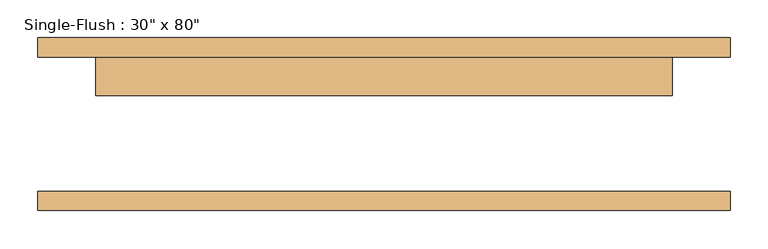
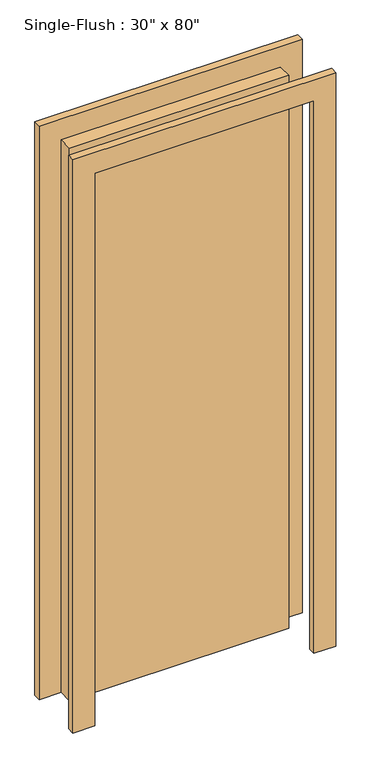
"""IFC4 building model written with IfcOpenShell, lengths in millimetres: door geometry."""

from ifc_helpers import new_model, si_unit, frame, origin, origin_with_axes, place, context, project, spatial, polyline, outline, extrude, source, transform, mapped, element, save


def door_41c6c2d7(model_context):
    return source(origin(), model_context, "Body", "SweptSolid", [
        extrude(outline(polyline([(2108.2, -457.2), (0.0, -457.2), (0.0, -381.0), (2032.0, -381.0), (2032.0, 381.0), (0.0, 381.0), (0.0, 457.2), (2108.2, 457.2), (2108.2, -457.2)])), frame((0.0, 88.9, 0.0), z_axis=(0.0, 1.0, 0.0), x_axis=(0.0, 0.0, 1.0)), (0.0, 0.0, 1.0), 25.4),
        extrude(outline(polyline([(2108.2, 457.2), (2108.2, -457.2), (0.0, -457.2), (0.0, -381.0), (2032.0, -381.0), (2032.0, 381.0), (0.0, 381.0), (0.0, 457.2), (2108.2, 457.2)])), frame((0.0, -114.3, 0.0), z_axis=(0.0, 1.0, 0.0), x_axis=(0.0, 0.0, 1.0)), (0.0, 0.0, 1.0), 25.4),
        extrude(outline(polyline([(381.0, 38.1), (-381.0, 38.1), (-381.0, 88.9), (381.0, 88.9), (381.0, 38.1)])), origin_with_axes(), (0.0, 0.0, 1.0), 2032.0),
    ])


if __name__ == "__main__":
    model = new_model("IFC4")
    model_context = context("Model", 3, world=origin())
    ifc_project = project(units=[si_unit("LENGTHUNIT", "METRE", prefix="MILLI")], contexts=[model_context])
    site = spatial("IfcSite", under=ifc_project)
    building = spatial("IfcBuilding", under=site)
    placement = place(None, origin())
    door_shape = door_41c6c2d7(model_context)
    element("IfcDoor", 1, ObjectType="Single-Flush : 30\" x 80\"", at=placement, inside=building, context=model_context, shape_type="MappedRepresentation", body=[
        mapped(door_shape, transform((0.0, 0.0, 0.0), x_axis=(1.0, 0.0, 0.0), y_axis=(0.0, 1.0, 0.0), z_axis=(0.0, 0.0, 1.0))),
    ])
    save(model, "model.ifc")

# Revit data of these elements
# Type "Single-Flush : 30\" x 80\""
#   Type Mark = "5"
#   Construction Type Id = "MDOOR"
#   Assembly Code = "C1020"
#   Analytic Construction = "Metal"
#   Thickness = 0' - 2"
#   Heat Transfer Coefficient (U) = 0.651978 BTU/(h·ft²·°F)
#   Height = 6' - 8"
#   Trim Projection Ext = 0' - 1"
#   Trim Projection Int = 0' - 1"
#   Trim Width = 0' - 3"
#   Width = 2' - 6"
#   Define Thermal Properties by = 1
#   Door Material = Door - Panel
#   Frame Material = Door - Frame
#   Visual Light Transmittance = 0
#   Solar Heat Gain Coefficient = 0
#   Function = (empty or 0)
#   Wall Closure = (empty or 0)
# Element 1 (IfcDoor, "Single-Flush : 30\" x 80\"")
#   Materials on its faces: "Door - Frame", "Door - Panel"
# Materials
#   "Door - Panel": class "Wood", colour RGB 210 159 95, transparency 0
#   "Door - Frame": colour RGB 118 70 51, transparency 0
